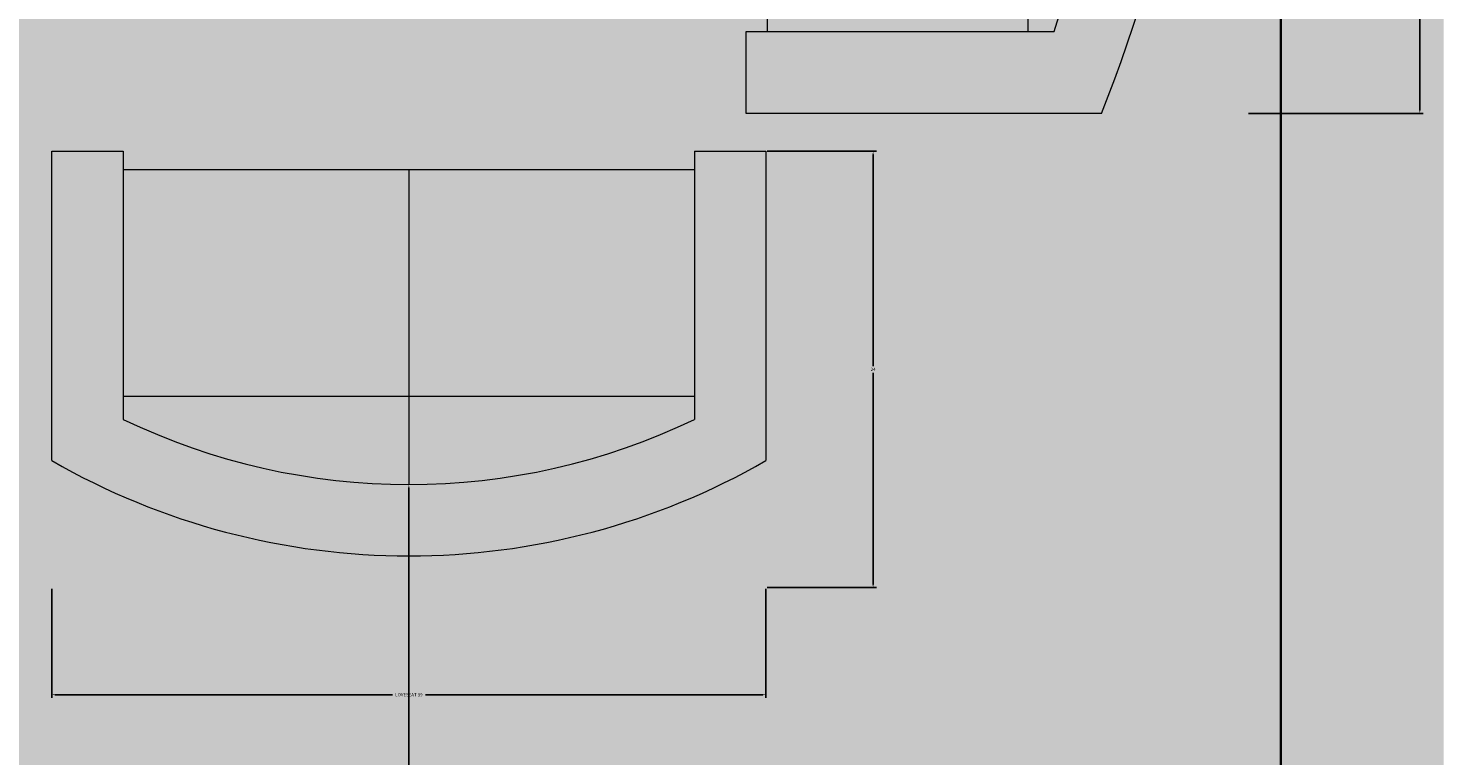
# Model space of a CAD drawing. Units: inches. Extents: x 3024 to 3952, y 1308 to 1863.
# Tile 13 of 29: x 3392 to 3469, y 1449 to 1489. Entities that reach past the tile are written whole.
import ezdxf

# ---------------------------------------------------------------- set-up
doc = ezdxf.new("R2010")
doc.units = ezdxf.units.IN
for name, color, linetype, lineweight in [('A-ANNO-DIMS', 2, 'Continuous', 18), ('A-FLOR-TILE-PATT', 7, 'Continuous', 13), ('A-FURN', 8, 'Continuous', 18), ('A-FURN-PATT', 9, 'Continuous', 13), ('A-WALL', 7, 'Continuous', 35)]:
    doc.layers.add(name, color=color, linetype=linetype, lineweight=lineweight)
doc.layers.add('A-FLOR-PATT', color=254, linetype='Continuous', lineweight=13, true_color=0xfeeab9)
doc.layers.add('A-WALL-PATT', color=254, linetype='Continuous', lineweight=13, true_color=0xcecce6)
doc.styles.get("Standard").update_dxf_attribs({"font": 'arial.ttf'})
doc.dimstyles.get("Standard").update_dxf_attribs({"dimtxt": 0.18, "dimasz": 0.18, "dimexe": 0.18, "dimexo": 0.0625, "dimgap": 0.09, "dimtad": 0, "dimtih": 1, "dimtoh": 1, "dimdec": 4, "dimzin": 0, "dimdsep": 46, "dimtxsty": 'Standard', "dimcen": 0.09, "dimadec": 0, "dimazin": 0, "dimtfac": 1, "dimtdec": 4, "dimtofl": 0, "dimtmove": 0, "dimatfit": 3, "dimfxl": 1, "dimtolj": 1, "dimtzin": 0, "dimarcsym": 0})

# ---------------------------------------------------------------- blocks, each defined once
blk = doc.blocks.new('Sofa - Roundback 7 ft.')
for p, q in [((-12.00002, -32.4421), (-12.00003, -6.5971)), ((11.99997, -32.4421), (11.99998, -6.5971)), ((-36.000027, -34), (-36.000027, -11.4696)), ((35.99998, -34), (35.99998, -11.4696)), ((-35.999844, -13.3819), (35.9998, -13.3819)), ((-36.000027, -32.4421), (35.99998, -32.4421))]:
    blk.add_line(p, q)
for points in [[(-36.000027, -34), (-42.000027, -34), (-42.000027, -8)], [(41.99998, -8), (41.99998, -34), (35.99998, -34)]]:
    blk.add_lwpolyline(points)
for centre, radius, start, end in [((0, -114.25), 114.25, 68.43141, 111.5686), ((-0.00001, -127.1968), 121.1968, 72.72033, 107.2797)]:
    blk.add_arc(centre, radius, start, end)
blk = doc.blocks.new('Sofa - Roundback Loveseat 5 ft.')
for p, q in [((0, -32.44198), (0, -5.99998)), ((-24, -33.99998), (-24, -11.46958)), ((24.00004, -33.99998), (24.00004, -11.46958)), ((-23.9998, -13.38178), (23.99986, -13.38178)), ((-24, -32.44198), (24.00004, -32.44198))]:
    blk.add_line(p, q)
for points in [[(-24, -33.99998), (-30, -33.99998), (-30, -7.99998)], [(30.00004, -7.99998), (30.00004, -33.99998), (24.00004, -33.99998)]]:
    blk.add_lwpolyline(points)
for centre, radius, start, end in [((0, -60.24998), 60.24998, 60.13715, 119.8628), ((0, -61.38438), 55.38444, 64.32083, 115.6792)]:
    blk.add_arc(centre, radius, start, end)
blk = doc.blocks.new('*D28')
at = {"layer": 'A-ANNO-DIMS', "color": 0, "lineweight": -2, "transparency": 16777216}
for p, q in [((3458.989, 1547.543), (3468.633, 1547.543)), ((3468.453, 1547.363), (3468.453, 1515.97)), ((3468.453, 1484.211), (3468.453, 1515.604)), ((3458.989, 1484.031), (3468.633, 1484.031))]:
    blk.add_line(p, q, dxfattribs=at)
at = {"layer": 'A-ANNO-DIMS', "color": 0, "transparency": 16777216}
for points in [[(3468.423, 1547.363), (3468.483, 1547.363), (3468.453, 1547.543)], [(3468.423, 1484.211), (3468.483, 1484.211), (3468.453, 1484.031)]]:
    blk.add_solid(points, dxfattribs=at)
at = {"layer": 'Defpoints', "color": 0, "transparency": 16777216}
for p in [(3458.926, 1547.543), (3458.926, 1484.031), (3468.453, 1484.031)]:
    blk.add_point(p, dxfattribs=at)
at = {"layer": 'A-ANNO-DIMS', "color": 0, "transparency": 16777216, "insert": (3468.453, 1515.787), "char_height": 0.18, "attachment_point": 5}
blk.add_mtext('\\A1;SOFA 64', dxfattribs=at)
blk = doc.blocks.new('*D30')
at = {"layer": 'A-ANNO-DIMS', "color": 0, "lineweight": -2, "transparency": 16777216}
for p, q in [((3392.822, 1457.753), (3392.822, 1451.713)), ((3432.307, 1457.753), (3432.307, 1451.713)), ((3393.002, 1451.893), (3411.651, 1451.893)), ((3432.127, 1451.893), (3413.478, 1451.893))]:
    blk.add_line(p, q, dxfattribs=at)
at = {"layer": 'A-ANNO-DIMS', "color": 0, "transparency": 16777216}
for points in [[(3393.002, 1451.923), (3393.002, 1451.863), (3392.822, 1451.893)], [(3432.127, 1451.923), (3432.127, 1451.863), (3432.307, 1451.893)]]:
    blk.add_solid(points, dxfattribs=at)
at = {"layer": 'Defpoints', "color": 0, "transparency": 16777216}
for p in [(3392.822, 1457.816), (3432.307, 1457.816), (3392.822, 1451.893)]:
    blk.add_point(p, dxfattribs=at)
at = {"layer": 'A-ANNO-DIMS', "color": 0, "transparency": 16777216, "insert": (3412.565, 1451.893), "char_height": 0.18, "attachment_point": 5}
blk.add_mtext('\\A1;LOVESEAT 39', dxfattribs=at)
blk = doc.blocks.new('*D31')
at = {"layer": 'A-ANNO-DIMS', "color": 0, "lineweight": -2, "transparency": 16777216}
for p, q in [((3432.369, 1481.945), (3438.41, 1481.945)), ((3438.23, 1481.765), (3438.23, 1470.061)), ((3438.23, 1457.996), (3438.23, 1469.7)), ((3432.369, 1457.816), (3438.41, 1457.816))]:
    blk.add_line(p, q, dxfattribs=at)
at = {"layer": 'A-ANNO-DIMS', "color": 0, "transparency": 16777216}
for points in [[(3438.2, 1481.765), (3438.26, 1481.765), (3438.23, 1481.945)], [(3438.2, 1457.996), (3438.26, 1457.996), (3438.23, 1457.816)]]:
    blk.add_solid(points, dxfattribs=at)
at = {"layer": 'Defpoints', "color": 0, "transparency": 16777216}
for p in [(3432.307, 1481.945), (3432.307, 1457.816), (3438.23, 1457.816)]:
    blk.add_point(p, dxfattribs=at)
at = {"layer": 'A-ANNO-DIMS', "color": 0, "transparency": 16777216, "insert": (3438.23, 1469.881), "char_height": 0.18, "attachment_point": 5}
blk.add_mtext('\\A1;24', dxfattribs=at)
blk = doc.blocks.new('*D107')
at = {"layer": 'A-ANNO-DIMS', "color": 0, "lineweight": -2, "transparency": 16777216}
for p, q in [((3412.475, 1499.22), (3412.655, 1499.22)), ((3412.565, 1499.13), (3412.565, 1499.31)), ((3412.565, 1435.781), (3412.565, 1459.391)), ((3412.745, 1435.781), (3412.565, 1435.781))]:
    blk.add_line(p, q, dxfattribs=at)
at = {"layer": 'A-ANNO-DIMS', "color": 0, "transparency": 16777216}
blk.add_solid([(3412.595, 1459.391), (3412.535, 1459.391), (3412.565, 1459.571)], dxfattribs=at)
at = {"layer": 'Defpoints', "color": 0, "transparency": 16777216}
for p in [(3412.565, 1499.22), (3412.565, 1459.571)]:
    blk.add_point(p, dxfattribs=at)
at = {"layer": 'A-ANNO-DIMS', "color": 0, "transparency": 16777216, "insert": (3413.226, 1435.781), "char_height": 0.18, "attachment_point": 5}
blk.add_mtext('\\A1;R39.65', dxfattribs=at)
blk = doc.blocks.new('*D108')
at = {"layer": 'A-ANNO-DIMS', "color": 0, "lineweight": -2, "transparency": 16777216}
for p, q in [((3412.475, 1499.966), (3412.655, 1499.966)), ((3412.565, 1499.876), (3412.565, 1500.056)), ((3412.565, 1441.651), (3412.565, 1463.339)), ((3412.745, 1441.651), (3412.565, 1441.651))]:
    blk.add_line(p, q, dxfattribs=at)
at = {"layer": 'A-ANNO-DIMS', "color": 0, "transparency": 16777216}
blk.add_solid([(3412.595, 1463.339), (3412.535, 1463.339), (3412.565, 1463.519)], dxfattribs=at)
at = {"layer": 'Defpoints', "color": 0, "transparency": 16777216}
for p in [(3412.565, 1499.966), (3412.565, 1463.519)]:
    blk.add_point(p, dxfattribs=at)
at = {"layer": 'A-ANNO-DIMS', "color": 0, "transparency": 16777216, "insert": (3413.226, 1441.651), "char_height": 0.18, "attachment_point": 5}
blk.add_mtext('\\A1;R36.45', dxfattribs=at)

msp = doc.modelspace()

# ---------------------------------------------------------------- hatches: boundary and pattern name
at = {"layer": 'A-FLOR-PATT', "transparency": 33554528}
h = msp.add_hatch(color=256, dxfattribs=at)
h.dxf.hatch_style = 1
h.paths.add_polyline_path([(3460.764, 1688.6064), (3412.764, 1688.6064), (3412.764, 1694.6064), (3460.764, 1694.6064), (3460.764, 1778.6064), (3406.764, 1778.6064), (3406.764, 1759.9514), (3318.2981, 1759.9514), (3318.2981, 1658.6064), (3322.5356, 1658.6064), (3322.5356, 1652.6064), (3292.764, 1652.6064), (3292.764, 1778.6064), (3106.764, 1778.6064), (3106.764, 1628.6064), (3172.764, 1628.6064), (3172.764, 1532.6064), (3166.764, 1532.6064), (3166.764, 1628.6064), (3106.764, 1628.6064), (3106.764, 1356.8452), (3202.812, 1356.8452), (3202.812, 1354.2534), (3202.812, 1353.8388), (3202.812, 1351.1212), (3202.812, 1347.8452), (3277.764, 1347.8452), (3277.764, 1353.8452), (3277.764, 1356.8452), (3277.764, 1442.6064), (3460.764, 1442.6064)])
h.paths.add_polyline_path([(3216.238, 1527.2064), (3216.238, 1491.2064), (3214.663, 1491.2064), (3214.663, 1491.2409, -0.3966224), (3180.243, 1526.6064), (3163.0285, 1526.6064), (3163.0285, 1531.1064), (3161.716, 1531.1064), (3161.716, 1561.1064), (3163.0285, 1561.1064), (3163.0285, 1531.1064), (3163.0285, 1526.6064), (3180.243, 1526.6064, 0.3966224), (3214.663, 1491.2409), (3214.663, 1527.2064)], flags=16)
h.paths.add_polyline_path([(3227.364, 1649.8972), (3191.364, 1649.8972), (3191.364, 1651.4722), (3227.364, 1651.4722)], flags=16)
h.paths.add_polyline_path([(3323.1172, 1606.7362), (3323.8545, 1606.8514), (3323.8545, 1594.8241), (3323.1172, 1594.9393)], flags=16)
h.paths.add_polyline_path([(3324.2232, 1606.909), (3330.1216, 1607.8307), (3330.1216, 1614.1093), (3339.3495, 1614.1093), (3340.2711, 1620.0078), (3352.4136, 1620.0078), (3353.3353, 1614.1093), (3359.9941, 1614.1093), (3360.9157, 1620.0078), (3373.0582, 1620.0078), (3373.9799, 1614.1093), (3383.2077, 1614.1093), (3383.2077, 1607.8307), (3389.1062, 1606.909), (3389.1062, 1594.7665), (3383.2077, 1593.8449), (3383.2077, 1587.5663), (3373.9799, 1587.5663), (3373.0583, 1581.6678), (3360.9157, 1581.6678), (3359.9941, 1587.5663), (3353.3353, 1587.5663), (3352.4136, 1581.6678), (3340.2711, 1581.6678), (3339.3495, 1587.5663), (3330.1216, 1587.5663), (3330.1216, 1593.8449), (3324.2232, 1594.7665)], flags=16)
h.paths.add_polyline_path([(3236.1584, 1693.1064), (3236.1584, 1723.1064), (3237.4709, 1723.1064), (3237.4709, 1693.1064)], flags=16)
h.paths.add_polyline_path([(3373.2158, 1600.6847), (3373.7965, 1600.7303), (3374.3268, 1600.7874), (3374.8132, 1600.8531), (3375.2621, 1600.9247), (3375.6801, 1600.9991), (3376.0736, 1601.0735), (3376.6855, 1601.19), (3377.366, 1601.3023), (3378.0667, 1601.3814), (3378.8026, 1601.4123), (3379.5865, 1601.3839), (3380.4537, 1601.2948), (3381.301, 1601.1717), (3382.0317, 1601.0433), (3382.4398, 1600.9607), (3382.6252, 1600.9201), (3382.919, 1600.8507), (3382.9044, 1600.8531), (3382.842, 1600.8678), (3382.7541, 1600.8896), (3382.6252, 1600.9201), (3382.4398, 1600.9607), (3382.1868, 1601.0119), (3381.8738, 1601.0711), (3381.5125, 1601.1346), (3381.1149, 1601.1988), (3380.6928, 1601.2601), (3380.2581, 1601.3149), (3379.8226, 1601.3597), (3379.3984, 1601.3908), (3378.9944, 1601.4054), (3378.6092, 1601.4042), (3378.2384, 1601.3886), (3377.8777, 1601.36), (3377.5227, 1601.32), (3377.1691, 1601.2698), (3376.8127, 1601.211), (3376.4491, 1601.145), (3376.0736, 1601.0735), (3375.4177, 1600.9494), (3374.5542, 1600.8119), (3373.5044, 1600.6988)], flags=0)
h.paths.add_polyline_path([(3380.0253, 1596.7351), (3380.499, 1596.6659), (3380.9706, 1596.6119), (3381.4375, 1596.5791), (3381.8971, 1596.5736), (3382.5886, 1596.6167), (3382.7848, 1596.6692), (3382.1465, 1596.5706), (3381.236, 1596.5815), (3380.3199, 1596.6865)], flags=0)
h.paths.add_polyline_path([(3369.6414, 1603.9617), (3370.1589, 1604.0021), (3370.6218, 1604.0539), (3371.0335, 1604.1173), (3371.3978, 1604.1921), (3371.7181, 1604.2785), (3371.9984, 1604.3761), (3372.2441, 1604.483), (3372.4611, 1604.5972), (3372.655, 1604.7163), (3372.8317, 1604.8384), (3372.9968, 1604.9611), (3373.3703, 1605.2455), (3373.8426, 1605.5328), (3374.4624, 1605.7539), (3375.1058, 1605.8302), (3375.7221, 1605.8261), (3376.4109, 1605.76), (3377.1534, 1605.6376), (3377.8945, 1605.473), (3378.1382, 1605.409), (3377.7394, 1605.5074), (3377.3509, 1605.5937), (3376.9704, 1605.6677), (3376.5999, 1605.7288), (3376.2417, 1605.7762), (3375.8979, 1605.8092), (3375.5707, 1605.8271), (3375.2621, 1605.8291), (3374.9745, 1605.8146), (3374.7092, 1605.7832), (3374.4647, 1605.7359), (3374.239, 1605.6742), (3374.0298, 1605.5996), (3373.835, 1605.5134), (3373.6525, 1605.4171), (3373.4801, 1605.3123), (3373.3156, 1605.2002), (3373.1562, 1605.0825), (3372.7603, 1604.781), (3372.236, 1604.4588), (3371.5738, 1604.2283), (3370.8493, 1604.0794), (3369.9262, 1603.976)], flags=0)
h.paths.add_polyline_path([(3366.7533, 1606.5832), (3367.1713, 1606.5519), (3367.5378, 1606.5374), (3367.8568, 1606.5394), (3368.1325, 1606.5573), (3368.3694, 1606.5903), (3368.5717, 1606.6377), (3368.7438, 1606.6988), (3368.89, 1606.7728), (3369.0146, 1606.8591), (3369.121, 1606.9568), (3369.2094, 1607.0646), (3369.2792, 1607.181), (3369.3295, 1607.3046), (3369.3596, 1607.4339), (3369.3688, 1607.5676), (3369.3565, 1607.7042), (3369.3218, 1607.8422), (3369.2649, 1607.9804), (3369.1893, 1608.1187), (3369.0993, 1608.2569), (3368.9992, 1608.3952), (3368.8934, 1608.5334), (3368.7861, 1608.6717), (3368.6817, 1608.8099), (3368.4212, 1609.1804), (3368.2685, 1609.7106), (3368.4883, 1610.1814), (3369.0537, 1610.4604), (3369.6717, 1610.5097), (3370.2812, 1610.3612), (3370.4805, 1610.2968), (3370.1882, 1610.3839), (3369.9284, 1610.4472), (3369.6905, 1610.4842), (3369.4662, 1610.4933), (3369.2555, 1610.4765), (3369.0608, 1610.4367), (3368.884, 1610.3767), (3368.7274, 1610.2994), (3368.5931, 1610.2077), (3368.4833, 1610.1045), (3368.4002, 1609.9927), (3368.3451, 1609.8747), (3368.3166, 1609.7517), (3368.3127, 1609.6244), (3368.331, 1609.4935), (3368.3696, 1609.3597), (3368.4261, 1609.2237), (3368.4985, 1609.0863), (3368.5845, 1608.9482), (3368.6817, 1608.8099), (3368.7861, 1608.6717), (3368.8934, 1608.5334), (3368.9992, 1608.3952), (3369.0993, 1608.2569), (3369.3398, 1607.8876), (3369.3941, 1607.2896), (3368.9774, 1606.7817), (3368.3928, 1606.5742), (3367.7162, 1606.5303), (3367.0044, 1606.5585)], flags=0)
h.paths.add_polyline_path([(3362.1859, 1610.2589), (3362.5478, 1610.2845), (3362.8348, 1610.3275), (3363.0585, 1610.3863), (3363.2303, 1610.4595), (3363.3619, 1610.5457), (3363.463, 1610.6432), (3363.5376, 1610.7502), (3363.5876, 1610.8643), (3363.6153, 1610.9834), (3363.6229, 1611.1055), (3363.6125, 1611.2283), (3363.5861, 1611.3496), (3363.5462, 1611.4673), (3363.4949, 1611.5797), (3363.4358, 1611.6871), (3363.3723, 1611.7902), (3363.3081, 1611.8897), (3363.2468, 1611.9863), (3363.192, 1612.0808), (3363.0258, 1612.4261), (3363.3371, 1612.8672), (3363.9008, 1612.9782), (3364.4822, 1612.9641), (3365.1098, 1612.9074), (3365.328, 1612.8805), (3364.9615, 1612.9208), (3364.6426, 1612.9496), (3364.3668, 1612.9669), (3364.1299, 1612.9726), (3363.9276, 1612.9669), (3363.7555, 1612.9496), (3363.6093, 1612.9208), (3363.4848, 1612.8805), (3363.3782, 1612.8289), (3363.2889, 1612.7672), (3363.2169, 1612.6969), (3363.1622, 1612.6193), (3363.1247, 1612.5361), (3363.1046, 1612.4484), (3363.1017, 1612.358), (3363.1161, 1612.266), (3363.1472, 1612.1738), (3363.192, 1612.0808), (3363.2468, 1611.9863), (3363.3081, 1611.8897), (3363.3723, 1611.7902), (3363.4358, 1611.6871), (3363.6363, 1611.323), (3363.5979, 1610.7003), (3363.0863, 1610.3651), (3362.3983, 1610.2622)], flags=0)
h.paths.add_polyline_path([(3352.356, 1581.2991), (3352.2408, 1580.5618), (3340.4439, 1580.5618), (3340.3287, 1581.2991)], flags=16)
h.paths.add_polyline_path([(3340.4439, 1621.1137), (3352.2408, 1621.1137), (3352.356, 1620.3764), (3340.3287, 1620.3764)], flags=16)
h.paths.add_polyline_path([(3278.4282, 1504.7424), (3290.3831, 1504.7424), (3290.3831, 1502.7499), (3291.0473, 1502.7499), (3291.0473, 1494.7799), (3290.3831, 1494.7799), (3290.3831, 1494.1158), (3291.0473, 1494.1158), (3291.0473, 1486.1458), (3290.3831, 1486.1458), (3290.3831, 1484.1533), (3291.0473, 1484.1533), (3291.0473, 1483.4892, -0.0909091), (3291.0473, 1468.8776), (3291.0473, 1468.2135), (3290.3831, 1468.2135), (3290.3831, 1464.8926), (3278.4282, 1464.8926), (3278.4282, 1472.8626), (3277.764, 1473.5268), (3277.764, 1478.84), (3278.4282, 1479.5042)], flags=16)
h.paths.add_polyline_path([(3278.7603, 1504.4103), (3290.051, 1504.4103), (3290.051, 1465.2247), (3278.7603, 1465.2247)], flags=0)
h.paths.add_polyline_path([(3123.904, 1600.7821), (3117.9039, 1602.7821), (3117.9039, 1599.7821), (3119.4039, 1599.7821), (3119.4039, 1596.7821), (3118.4039, 1596.7821), (3118.4039, 1598.7821), (3117.9039, 1598.7821), (3117.9039, 1596.2821), (3109.9039, 1596.2821), (3109.9039, 1617.2821), (3117.9039, 1617.2821), (3117.9039, 1610.7821), (3123.9038, 1612.7821, -0.7025712), (3137.9039, 1606.7822, -0.7025621)], flags=16)
h.paths.add_polyline_path([(3123.9039, 1602.7822), (3123.9039, 1610.7822, -0.7345333), (3136.9039, 1606.7822, -0.7345297)], flags=0)
h.paths.add_polyline_path([(3177.972, 1689.6473), (3109.2405, 1689.6473), (3109.2405, 1741.1959), (3177.972, 1741.1959)], flags=16)
h.paths.add_polyline_path([(3373.0006, 1581.2991), (3372.8854, 1580.5618), (3361.0885, 1580.5618), (3360.9733, 1581.2991)], flags=16)
h.paths.add_polyline_path([(3361.0885, 1621.1137), (3372.8854, 1621.1137), (3373.0006, 1620.3764), (3360.9733, 1620.3764)], flags=16)
h.paths.add_polyline_path([(3116.9039, 1598.2821, -0.4142136), (3116.1539, 1597.2821), (3111.9039, 1597.2821, -0.4142136), (3110.9039, 1598.0321), (3110.9039, 1615.2821, -0.4142136), (3111.6539, 1616.2821), (3115.9039, 1616.2821, -0.4142136), (3116.9039, 1615.5321)], flags=0)
h.paths.add_polyline_path([(3121.6122, 1728.1369), (3121.6122, 1696.5205), (3110.2715, 1696.5205), (3110.2715, 1714.3906), (3121.6122, 1714.3906), (3121.6122, 1716.4526), (3110.2715, 1716.4526), (3110.2715, 1734.3228), (3123.3304, 1734.3228), (3123.3304, 1729.8552), (3134.6711, 1741.1959), (3134.6711, 1728.1369)], flags=0)
h.paths.add_polyline_path([(3389.4748, 1606.8514), (3390.2122, 1606.7362), (3390.2122, 1594.9393), (3389.4748, 1594.8241)], flags=16)
h.paths.add_polyline_path([(3257.6842, 1762.8281), (3259.6842, 1768.8281), (3256.6842, 1768.8281), (3256.6842, 1767.3281), (3253.6842, 1767.3281), (3253.6842, 1768.3281), (3255.6842, 1768.3281), (3255.6842, 1768.8281), (3253.1842, 1768.8281), (3253.1842, 1776.8281), (3274.1842, 1776.8281), (3274.1842, 1768.8281), (3267.6842, 1768.8281), (3269.6842, 1762.8282, -0.7025712), (3263.6843, 1748.8282, -0.7025621)], flags=16)
h.paths.add_polyline_path([(3259.6842, 1762.8281), (3267.6843, 1762.8281, -0.7345333), (3263.6842, 1749.8282, -0.7345297)], flags=0)
h.paths.add_polyline_path([(3411.264, 1715.6064), (3411.264, 1716.9189), (3441.264, 1716.9189), (3441.264, 1715.6064)], flags=16)
h.paths.add_polyline_path([(3178.3806, 1449.1876), (3178.3806, 1397.639), (3109.6491, 1397.639), (3109.6491, 1449.1876)], flags=16)
h.paths.add_polyline_path([(3397.1501, 1541.7146), (3419.6183, 1541.7146), (3419.6183, 1496.7783), (3397.1501, 1496.7783)], flags=16)
h.paths.add_polyline_path([(3254.1842, 1770.5781), (3254.1842, 1774.8281, -0.4142136), (3254.9342, 1775.8281), (3272.1842, 1775.8281, -0.4142136), (3273.1842, 1775.0781), (3273.1842, 1770.8281, -0.4142136), (3272.4342, 1769.8281), (3255.1842, 1769.8281, -0.4142136)], flags=0)
h.paths.add_polyline_path([(3403.672, 1500.7601), (3403.6016, 1500.3997), (3403.5328, 1500.0441), (3403.4662, 1499.6867), (3403.4027, 1499.3226), (3403.3464, 1498.9532), (3403.3025, 1498.5811), (3403.2759, 1498.2091), (3403.2714, 1497.8401), (3403.3064, 1497.2813), (3403.3491, 1497.1219), (3403.2689, 1497.6395), (3403.2778, 1498.3719), (3403.3635, 1499.0984), (3403.4889, 1499.8168), (3403.6016, 1500.3997), (3403.672, 1500.7601), (3403.744, 1501.1315), (3403.817, 1501.5205), (3403.891, 1501.9336), (3403.9656, 1502.3769), (3404.0404, 1502.8572), (3404.115, 1503.3786), (3404.2264, 1504.2311), (3404.2571, 1504.5223), (3404.1552, 1503.6598), (3404.0063, 1502.6193), (3403.8604, 1501.7518), (3403.744, 1501.1315)], flags=0)
h.paths.add_polyline_path([(3406.5868, 1505.0416), (3406.6121, 1504.5236), (3406.6492, 1504.0526), (3406.6956, 1503.624), (3406.7491, 1503.2333), (3406.8072, 1502.8759), (3406.8676, 1502.5473), (3406.9281, 1502.243), (3407.0268, 1501.7597), (3407.1416, 1501.1368), (3407.2087, 1500.3904), (3407.1804, 1499.6703), (3407.1078, 1498.9956), (3407.0074, 1498.3199), (3406.8809, 1497.6059), (3406.7403, 1496.9627), (3406.7418, 1496.9824), (3406.7491, 1497.0249), (3406.8229, 1497.3409), (3406.8364, 1497.4025), (3406.878, 1497.6078), (3406.9261, 1497.8614), (3406.9777, 1498.1526), (3407.0298, 1498.4712), (3407.0797, 1498.8068), (3407.1243, 1499.149), (3407.1607, 1499.4874), (3407.1859, 1499.8115), (3407.1978, 1500.1137), (3407.1969, 1500.3962), (3407.1841, 1500.6642), (3407.1609, 1500.9225), (3407.1284, 1501.1761), (3407.0876, 1501.43), (3407.0398, 1501.6891), (3406.9862, 1501.9585), (3406.8832, 1502.4628), (3406.7712, 1503.0713), (3406.6657, 1503.8424), (3406.5924, 1504.7735)], flags=0)
h.paths.add_polyline_path([(3409.2517, 1507.8962), (3409.2752, 1507.4282), (3409.3079, 1507.0076), (3409.3501, 1506.6314), (3409.4015, 1506.2969), (3409.4624, 1506.0009), (3409.5326, 1505.7406), (3409.6119, 1505.5128), (3409.6988, 1505.3131), (3409.7915, 1505.1368), (3409.8883, 1504.9792), (3409.9875, 1504.8356), (3410.0872, 1504.7015), (3410.1859, 1504.572), (3410.4508, 1504.2132), (3410.7205, 1503.6035), (3410.8059, 1502.8824), (3410.7619, 1502.0875), (3410.6122, 1501.2299), (3410.4402, 1500.6169), (3410.2538, 1500.0031), (3410.0536, 1499.3219), (3409.9909, 1499.0812), (3410.1761, 1499.7472), (3410.3596, 1500.3513), (3410.4512, 1500.6561), (3410.5312, 1500.9412), (3410.6013, 1501.226), (3410.6614, 1501.512), (3410.7111, 1501.7964), (3410.7496, 1502.0763), (3410.7764, 1502.3489), (3410.7909, 1502.6114), (3410.7926, 1502.8608), (3410.7808, 1503.0944), (3410.7553, 1503.31), (3410.7169, 1503.5087), (3410.6667, 1503.6921), (3410.6061, 1503.8621), (3410.5361, 1504.0203), (3410.4578, 1504.1686), (3410.3726, 1504.3088), (3410.2815, 1504.4424), (3410.1859, 1504.572), (3410.0872, 1504.7015), (3409.859, 1505.0083), (3409.5943, 1505.5117), (3409.4266, 1506.1336), (3409.324, 1506.8011), (3409.2586, 1507.6407)], flags=0)
h.paths.add_polyline_path([(3411.4914, 1510.5878), (3411.4432, 1510.1586), (3411.4054, 1509.775), (3411.38, 1509.4354), (3411.3681, 1509.1376), (3411.3698, 1508.8784), (3411.3843, 1508.6542), (3411.4112, 1508.4618), (3411.4497, 1508.2974), (3411.4994, 1508.1575), (3411.5595, 1508.0388), (3411.6296, 1507.9375), (3411.7097, 1507.851), (3411.802, 1507.7792), (3411.9096, 1507.7225), (3412.0353, 1507.6817), (3412.1821, 1507.6572), (3412.3528, 1507.6496), (3412.5505, 1507.6597), (3412.778, 1507.6879), (3413.0364, 1507.7341), (3413.3194, 1507.7955), (3413.6188, 1507.8687), (3413.9264, 1507.95), (3414.234, 1508.036), (3414.5333, 1508.1232), (3414.8163, 1508.208), (3415.0747, 1508.287), (3415.3023, 1508.3569), (3415.5007, 1508.4158), (3415.6733, 1508.4617), (3416.1158, 1508.5538), (3416.512, 1508.2591), (3416.716, 1507.6581), (3416.61, 1507.0003), (3416.3052, 1506.3411), (3415.8928, 1505.618), (3415.7339, 1505.3633), (3415.9914, 1505.791), (3416.201, 1506.1583), (3416.3666, 1506.4739), (3416.4925, 1506.7462), (3416.5828, 1506.9838), (3416.6413, 1507.1949), (3416.6725, 1507.3883), (3416.6799, 1507.5705), (3416.6662, 1507.7417), (3416.6339, 1507.9), (3416.5851, 1508.0436), (3416.5223, 1508.1709), (3416.4478, 1508.28), (3416.3639, 1508.3692), (3416.273, 1508.4368), (3416.1765, 1508.4815), (3416.0718, 1508.5047), (3415.9553, 1508.5079), (3415.8237, 1508.493), (3415.6733, 1508.4617), (3415.5007, 1508.4158), (3415.3327, 1508.3659), (3414.6495, 1508.157), (3414.0606, 1507.9855), (3413.4456, 1507.8229), (3412.8838, 1507.701), (3412.5505, 1507.6597), (3412.0748, 1507.6354), (3411.595, 1507.8883), (3411.398, 1508.4429), (3411.3624, 1508.9927), (3411.3854, 1509.5711), (3411.4578, 1510.3071)], flags=0)
h.paths.add_polyline_path([(3135.0797, 1449.1876), (3135.0797, 1436.1286), (3122.0208, 1436.1286), (3122.0208, 1404.5122), (3110.6801, 1404.5122), (3110.6801, 1422.3823), (3122.0208, 1422.3823), (3122.0208, 1424.4443), (3110.6801, 1424.4443), (3110.6801, 1442.3145), (3123.739, 1442.3145), (3123.739, 1437.8469)], flags=0)
h.paths.add_polyline_path([(3416.4944, 1514.2949), (3416.4837, 1513.8511), (3416.4893, 1513.4867), (3416.5102, 1513.1926), (3416.5451, 1512.9593), (3416.5929, 1512.7775), (3416.6524, 1512.6379), (3416.7224, 1512.531), (3416.8017, 1512.4488), (3416.8886, 1512.3882), (3416.9813, 1512.3476), (3417.0781, 1512.3251), (3417.1773, 1512.3189), (3417.277, 1512.3274), (3417.3757, 1512.3488), (3417.4713, 1512.3813), (3417.5627, 1512.4229), (3417.65, 1512.471), (3417.7338, 1512.5225), (3417.8146, 1512.5747), (3417.8931, 1512.6245), (3417.9699, 1512.6691), (3418.2968, 1512.8265), (3418.6505, 1512.4645), (3418.7037, 1511.9342), (3418.6693, 1511.3839), (3418.6076, 1510.8228), (3418.5777, 1510.5927), (3418.6197, 1510.9333), (3418.6525, 1511.2311), (3418.6759, 1511.4903), (3418.6899, 1511.7144), (3418.6946, 1511.9069), (3418.6899, 1512.0713), (3418.6759, 1512.2112), (3418.6525, 1512.33), (3418.6197, 1512.4311), (3418.5778, 1512.5177), (3418.5276, 1512.5903), (3418.4705, 1512.6488), (3418.4075, 1512.6933), (3418.3399, 1512.7237), (3418.2686, 1512.7401), (3418.1951, 1512.7424), (3418.1204, 1512.7307), (3418.0455, 1512.7055), (3417.9792, 1512.6736), (3417.65, 1512.471), (3417.5627, 1512.4229), (3417.4713, 1512.3813), (3417.3757, 1512.3488), (3417.277, 1512.3274), (3416.878, 1512.2936), (3416.5757, 1512.7549), (3416.492, 1513.3145), (3416.4808, 1514.0384)], flags=0)
h.paths.add_polyline_path([(3392.8223, 1481.9454), (3396.7707, 1481.9454), (3396.7707, 1480.9201), (3428.3585, 1480.9201), (3428.3585, 1481.9454), (3432.3069, 1481.9454), (3432.3069, 1464.8354, -0.266667), (3392.8223, 1464.8354)], flags=16)
h.paths.add_polyline_path([(3431.203, 1547.5428), (3450.8613, 1547.5428, -0.1904762), (3450.8614, 1484.031), (3431.203, 1484.031), (3431.203, 1488.5675), (3432.3809, 1488.5675), (3432.3809, 1543.0062), (3431.203, 1543.0062)], flags=16)
h.paths.add_polyline_path([(3451.9233, 1524.86, -0.0496282), (3451.9233, 1506.7138), (3446.7921, 1506.7138), (3446.7921, 1524.86)], flags=0)
h.paths.add_polyline_path([(3460.764, 1436.6064), (3277.764, 1436.6064), (3277.764, 1356.8452), (3277.764, 1353.8452), (3460.764, 1353.8452)], flags=17)
h.paths.add_polyline_path([(3121.3033, 1577.378), (3153.693, 1577.378), (3153.693, 1586.6752), (3121.3033, 1586.6752)], flags=24)
h.paths.add_polyline_path([(3164.1457, 1464.1276), (3210.4801, 1464.1276), (3210.4801, 1473.4247), (3164.1457, 1473.4247)], flags=24)
h.paths.add_polyline_path([(3343.1909, 1505.8863), (3373.7236, 1505.8863), (3373.7236, 1515.1773), (3343.1909, 1515.1773)], flags=24)
h.paths.add_polyline_path([(3337.6353, 1564.2926), (3370.0189, 1564.2926), (3370.0189, 1573.5836), (3337.6353, 1573.5836)], flags=24)
h.paths.add_polyline_path([(3419.204, 1753.8578), (3453.3997, 1753.8578), (3453.3997, 1762.9956), (3419.204, 1762.9956)], flags=24)
h.paths.add_polyline_path([(3341.2523, 1701.0246), (3381.0761, 1701.0246), (3381.0761, 1710.3156), (3341.2523, 1710.3156)], flags=24)
h.paths.add_polyline_path([(3245.8895, 1726.2997), (3278.2793, 1726.2997), (3278.2793, 1735.5968), (3245.8895, 1735.5968)], flags=24)
h.paths.add_polyline_path([(3128.8045, 1668.6736), (3175.1389, 1668.6736), (3175.1389, 1677.9707), (3128.8045, 1677.9707)], flags=24)
h.paths.add_polyline_path([(3345.9997, 1396.0062), (3389.09, 1396.0062), (3389.09, 1405.3033), (3345.9997, 1405.3033)], flags=24)
at = {"layer": 'A-FLOR-TILE-PATT', "transparency": 33554569}
h = msp.add_hatch(dxfattribs=at)
h.set_pattern_fill('ANGLE', color=256, scale=2)
h.set_pattern_definition([(0, (0, 0), (0, 13.97), [10.16, -3.81]), (90, (0, 0), (-13.97, 9e-16), [10.16, -3.81])])
h.paths.add_polyline_path([(3292.764, 1778.6064), (3232.764, 1778.6064), (3232.764, 1694.6064), (3236.1584, 1694.6064), (3236.1584, 1723.1064), (3237.4709, 1723.1064), (3237.4709, 1723.0777, -0.3870039), (3266.1209, 1694.6064), (3292.764, 1694.6064)])
h.paths.add_polyline_path([(3263.6843, 1748.8282, -0.7025621), (3257.6842, 1762.8281), (3259.6842, 1768.8281), (3256.6842, 1768.8281), (3256.6842, 1767.3281), (3253.6842, 1767.3281), (3253.6842, 1768.3281), (3255.6842, 1768.3281), (3255.6842, 1768.8281), (3253.1842, 1768.8281), (3253.1842, 1776.8281), (3274.1842, 1776.8281), (3274.1842, 1768.8281), (3267.6842, 1768.8281), (3269.6842, 1762.8282, -0.7025712)], flags=16)
h.paths.add_polyline_path([(3263.6842, 1749.8282, -0.7345297), (3259.6842, 1762.8281), (3267.6843, 1762.8281, -0.7345333)], flags=0)
h.paths.add_polyline_path([(3255.1842, 1769.8281, -0.4142136), (3254.1842, 1770.5781), (3254.1842, 1774.8281, -0.4142136), (3254.9342, 1775.8281), (3272.1842, 1775.8281, -0.4142136), (3273.1842, 1775.0781), (3273.1842, 1770.8281, -0.4142136), (3272.4342, 1769.8281)], flags=0)
h.paths.add_polyline_path([(3460.764, 1436.6064), (3277.764, 1436.6064), (3277.764, 1356.8452), (3277.764, 1353.8452), (3460.764, 1353.8452)])
h.paths.add_polyline_path([(3166.764, 1628.6064), (3106.764, 1628.6064), (3106.764, 1532.6064), (3133.066, 1532.6064, -0.3870039), (3161.716, 1561.0777), (3161.716, 1561.1064), (3163.0285, 1561.1064), (3163.0285, 1532.6064), (3166.764, 1532.6064)])
h.paths.add_polyline_path([(3123.904, 1600.7821), (3117.9039, 1602.7821), (3117.9039, 1599.7821), (3119.4039, 1599.7821), (3119.4039, 1596.7821), (3118.4039, 1596.7821), (3118.4039, 1598.7821), (3117.9039, 1598.7821), (3117.9039, 1596.2821), (3109.9039, 1596.2821), (3109.9039, 1617.2821), (3117.9039, 1617.2821), (3117.9039, 1610.7821), (3123.9038, 1612.7821, -0.7025712), (3137.9039, 1606.7822, -0.7025621)], flags=16)
h.paths.add_polyline_path([(3123.9039, 1602.7822), (3123.9039, 1610.7822, -0.7345333), (3136.9039, 1606.7822, -0.7345297)], flags=0)
h.paths.add_polyline_path([(3116.1539, 1597.2821), (3111.9039, 1597.2821, -0.4142136), (3110.9039, 1598.0321), (3110.9039, 1615.2821, -0.4142136), (3111.6539, 1616.2821), (3115.9039, 1616.2821, -0.4142136), (3116.9039, 1615.5321), (3116.9039, 1598.2821, -0.4142136)], flags=0)
h.paths.add_polyline_path([(3245.8895, 1726.2997), (3278.2793, 1726.2997), (3278.2793, 1735.5968), (3245.8895, 1735.5968)], flags=24)
h.paths.add_polyline_path([(3345.9997, 1396.0062), (3389.09, 1396.0062), (3389.09, 1405.3033), (3345.9997, 1405.3033)], flags=24)
h.paths.add_polyline_path([(3121.3033, 1577.378), (3153.693, 1577.378), (3153.693, 1586.6752), (3121.3033, 1586.6752)], flags=24)
at = {"layer": 'A-FURN-PATT', "transparency": 33554600}
h = msp.add_hatch(color=256, dxfattribs=at)
h.dxf.hatch_style = 1
h.paths.add_polyline_path([(3450.8613, 1547.5428), (3431.203, 1547.5428), (3431.203, 1543.0062), (3448.2376, 1543.0062, -0.1519478), (3448.2376, 1488.5675), (3431.203, 1488.5675), (3431.203, 1484.031), (3450.8614, 1484.031, 0.1904762)])
h.paths.add_polyline_path([(3446.7921, 1543.0062), (3432.3809, 1543.0062), (3432.3809, 1524.86), (3446.7921, 1524.86)], flags=17)
h.paths.add_polyline_path([(3448.2376, 1543.0062), (3446.7921, 1543.0062), (3446.7921, 1524.86), (3451.9233, 1524.86, 0.0506466)], flags=17)
h.paths.add_polyline_path([(3446.7921, 1524.86), (3432.3809, 1524.86), (3432.3809, 1506.7138), (3446.7921, 1506.7138)], flags=17)
h.paths.add_polyline_path([(3451.9233, 1524.86), (3446.7921, 1524.86), (3446.7921, 1506.7138), (3451.9233, 1506.7138, 0.0496282)], flags=17)
h.paths.add_polyline_path([(3446.7921, 1506.7138), (3432.3809, 1506.7138), (3432.3809, 1488.5675), (3446.7921, 1488.5675)], flags=17)
h.paths.add_polyline_path([(3451.9233, 1506.7138), (3446.7921, 1506.7138), (3446.7921, 1488.5675), (3448.2376, 1488.5675, 0.0506467)], flags=17)
h.paths.add_polyline_path([(3428.3585, 1480.9201), (3412.5646, 1480.9201), (3412.5646, 1468.377), (3428.3585, 1468.377)], flags=17)
h.paths.add_polyline_path([(3412.5646, 1480.9201), (3396.7707, 1480.9201), (3396.7707, 1468.377), (3412.5646, 1468.377)], flags=17)
h.paths.add_polyline_path([(3396.7707, 1481.9454), (3392.8223, 1481.9454), (3392.8223, 1464.8354, 0.266667), (3432.3069, 1464.8354), (3432.3069, 1481.9454), (3428.3585, 1481.9454), (3428.3585, 1467.119, -0.2279232), (3396.7707, 1467.119)])
h.paths.add_polyline_path([(3428.3585, 1467.119), (3428.3585, 1468.377), (3412.5646, 1468.377), (3412.5646, 1463.5192, 0.1125187)], flags=17)
h.paths.add_polyline_path([(3412.5646, 1468.377), (3396.7707, 1468.377), (3396.7707, 1467.119, 0.1125189), (3412.5646, 1463.5192)], flags=17)
at = {"layer": 'A-WALL-PATT'}
h = msp.add_hatch(color=256, dxfattribs=at)
h.dxf.hatch_style = 1
h.paths.add_polyline_path([(3106.764, 1778.6064), (3140.5977, 1778.6064), (3140.5977, 1781.8824), (3140.5977, 1784.6), (3140.5977, 1787.6064), (3097.764, 1787.6064), (3097.764, 1590.213), (3101.04, 1590.213), (3103.7576, 1590.213), (3106.764, 1590.213)])
h.paths.add_polyline_path([(3253.5314, 1781.8824), (3253.5314, 1784.6), (3253.5314, 1787.6064), (3194.6826, 1787.6064), (3194.6826, 1785.0146), (3194.6826, 1784.6), (3194.6826, 1781.8824), (3194.6826, 1778.6064), (3253.5314, 1778.6064)])
h.paths.add_polyline_path([(3333.856, 1782.2838), (3333.856, 1784.7474), (3333.856, 1787.6064), (3272.0523, 1787.6064), (3272.0523, 1785.0146), (3272.0523, 1784.6), (3272.0523, 1781.8824), (3272.0523, 1778.6064), (3333.856, 1778.6064)])
h.paths.add_polyline_path([(3428.8344, 1784.6), (3428.8344, 1787.6064), (3378.3947, 1787.6064), (3378.3947, 1784.7474), (3378.3947, 1782.2838), (3378.3947, 1778.6064), (3428.8344, 1778.6064), (3428.8344, 1781.8824)], flags=17)
h.paths.add_polyline_path([(3469.764, 1787.6064), (3451.9386, 1787.6064), (3451.9386, 1785.0146), (3451.9386, 1784.6), (3451.9386, 1781.8824), (3451.9386, 1778.6064), (3460.764, 1778.6064), (3460.764, 1353.8452), (3277.764, 1353.8452), (3277.764, 1347.8452), (3469.764, 1347.8452), (3469.764, 1353.8452)])
h.paths.add_polyline_path([(3106.764, 1571.6922), (3104.1722, 1571.6922), (3103.7576, 1571.6922), (3101.04, 1571.6922), (3097.764, 1571.6922), (3097.764, 1347.8452), (3148.7271, 1347.8452), (3148.7271, 1351.1212), (3148.7271, 1353.8388), (3148.7271, 1356.8452), (3106.764, 1356.8452)])
h.paths.add_polyline_path([(3277.764, 1532.6064), (3262.7605, 1532.6064), (3262.7605, 1582.9359), (3256.7605, 1582.9359), (3256.7605, 1532.6064), (3244.2116, 1532.6064), (3216.238, 1532.6064), (3216.238, 1527.2064), (3216.238, 1526.6064), (3271.764, 1526.6064), (3271.764, 1356.8452), (3202.812, 1356.8452), (3202.812, 1354.2534), (3202.812, 1353.8388), (3202.812, 1351.1212), (3202.812, 1347.8452), (3277.764, 1347.8452), (3277.764, 1353.8452), (3277.764, 1356.8452)])
h.paths.add_polyline_path([(3180.238, 1532.6064), (3163.0285, 1532.6064), (3163.0285, 1531.1064), (3163.0285, 1526.6064), (3180.243, 1526.6064, -0.0041669), (3180.238, 1527.2064)])
h.paths.add_polyline_path([(3133.0285, 1531.1064, -0.0125059), (3133.066, 1532.6064), (3106.764, 1532.6064), (3106.764, 1526.6064), (3133.0285, 1526.6064)], flags=17)
h.paths.add_polyline_path([(3172.764, 1628.6064), (3166.764, 1628.6064), (3166.764, 1532.6064), (3172.764, 1532.6064)])
h.paths.add_polyline_path([(3232.764, 1649.8972), (3227.364, 1649.8972), (3226.764, 1649.8972), (3226.764, 1634.6064), (3106.764, 1634.6064), (3106.764, 1628.6064), (3232.764, 1628.6064)])

# ---------------------------------------------------------------- linework, layer by layer
at = {"layer": 'A-WALL'}
msp.add_line((3460.764, 1353.8452), (3460.764, 1778.6064), dxfattribs=at)

# ---------------------------------------------------------------- block references
at = {"layer": 'A-FURN'}
for name, p, xscale, yscale, zscale, rotation in [('Sofa - Roundback 7 ft.', (3456.9101, 1515.7869), 0.75609235024942, 0.75609235024942, 0.75609235024942, 270), ('Sofa - Roundback Loveseat 5 ft.', (3412.5646, 1459.5708), 0.6580774779001581, 0.6580774779001581, 0.6580774779001581, 180)]:
    msp.add_blockref(name, p, dxfattribs=dict(at, xscale=xscale, yscale=yscale, zscale=zscale, rotation=rotation))

# ---------------------------------------------------------------- dimensions: what is measured, and where the dimension line sits
at = {"layer": 'A-ANNO-DIMS'}
for base, p1, p2, angle, text, picture, middle in [((3468.4531, 1484.031), (3458.9263, 1547.5428), (3458.9263, 1484.031), 270, 'SOFA <>', '*D28', (3468.4531, 1515.7869)), ((3392.8223, 1451.8932), (3432.3069, 1457.8159), (3392.8223, 1457.8159), 180, 'LOVESEAT <>', '*D30', (3412.5646, 1451.8932))]:
    dim = msp.add_linear_dim(base=base, p1=p1, p2=p2, angle=angle, text=text, dimstyle='Standard', override={"dimdec": 0, "dimlfac": 1, "dimrnd": 0, "dimzin": 0, "dimdsep": 46, "dimlunit": 2}, dxfattribs=at)
    dim.commit()
    dim.dimension.update_dxf_attribs({"geometry": picture, "text_midpoint": middle})
for center, mpoint, picture, middle in [((3412.5646, 1499.9664), (3412.565, 1463.5192), '*D108', (3413.2257, 1441.6508)), ((3412.5646, 1499.2199), (3412.565, 1459.5708), '*D107', (3413.2257, 1435.7813))]:
    dim = msp.add_radius_dim(center=center, mpoint=mpoint, dimstyle='Standard', override={"dimdec": 2, "dimlfac": 1, "dimrnd": 0, "dimzin": 0, "dimdsep": 46, "dimlunit": 2}, dxfattribs=at)
    dim.commit()
    dim.dimension.update_dxf_attribs({"geometry": picture, "text_midpoint": middle, "dimtype": 164})
dim = msp.add_linear_dim(base=(3438.2296, 1457.8159), p1=(3432.3069, 1481.9454), p2=(3432.3069, 1457.8159), angle=270, dimstyle='Standard', override={"dimdec": 0, "dimlfac": 1, "dimrnd": 0, "dimzin": 0, "dimdsep": 46, "dimlunit": 2}, dxfattribs=at)
dim.commit()
dim.dimension.update_dxf_attribs({"geometry": '*D31', "text_midpoint": (3438.2296, 1469.8806)})

doc.saveas('drawing.dxf')
